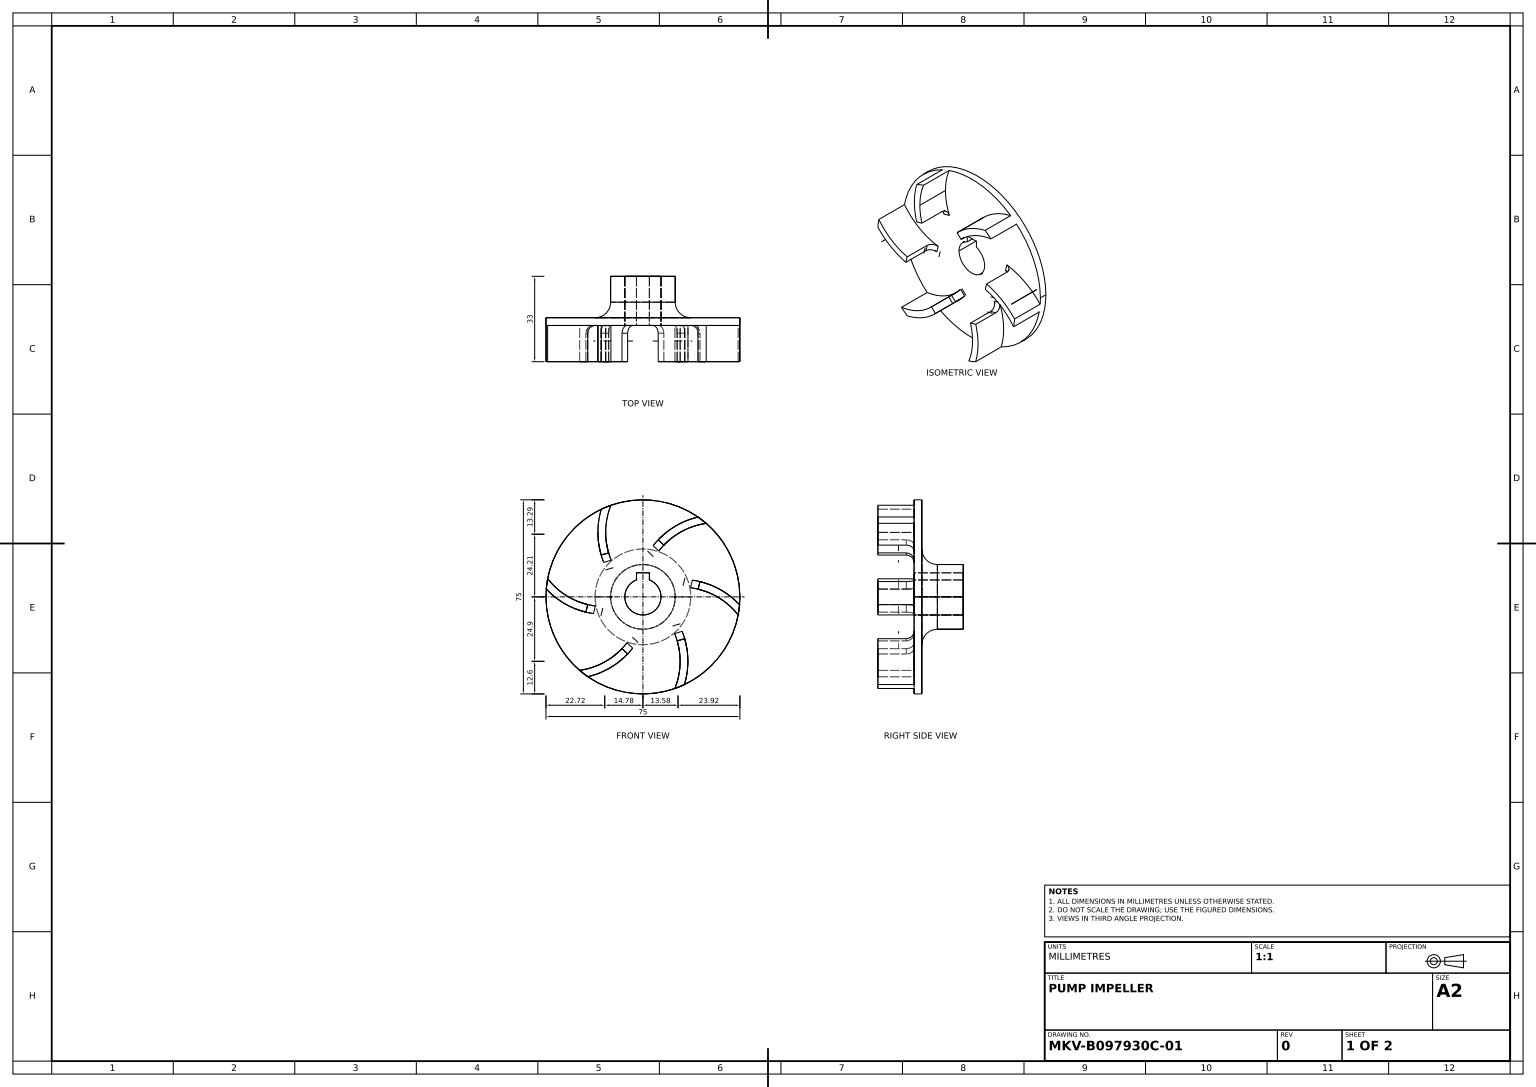
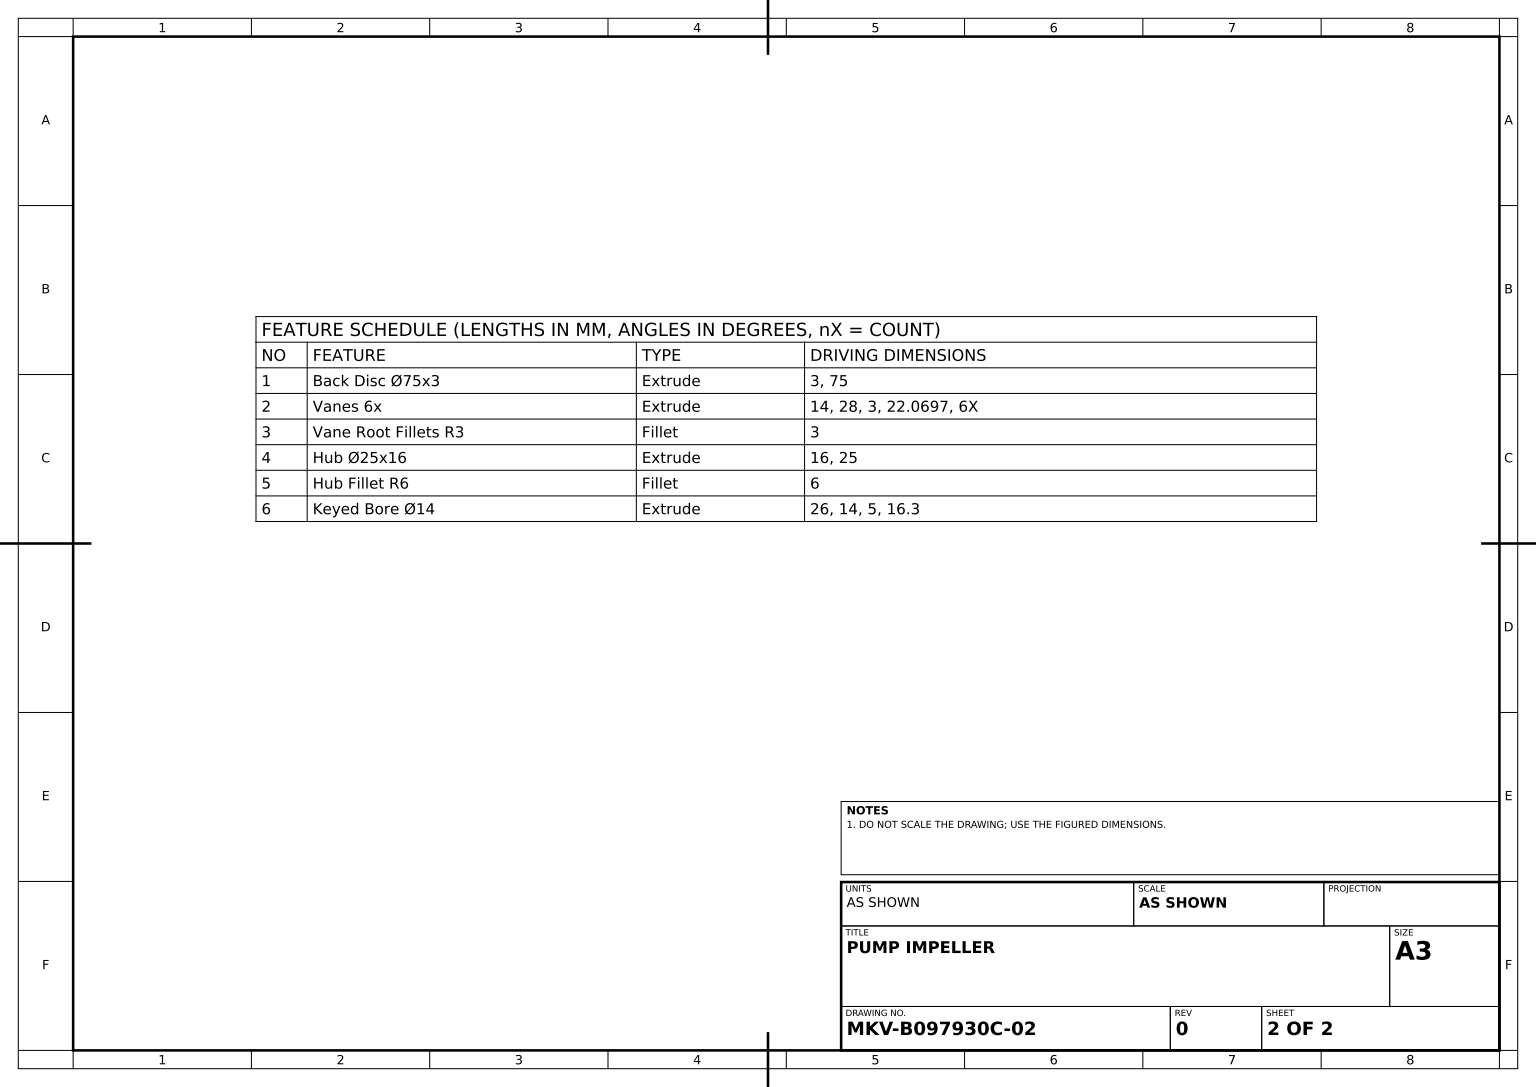
SolidWorks part; units mm, degrees
material "Plain Carbon Steel"
ref_plane "Front Plane" through (0, 0, 0) normal (0, 0, 1) x (1, 0, 0)
ref_plane "Top Plane" through (0, 0, 0) normal (0, 1, 0) x (1, 0, 0)
ref_plane "Right Plane" through (0, 0, 0) normal (1, 0, 0) x (0, 0, -1)
sketch "Back Disc Sketch Ø75" plane through (0, 0, 0) normal (0, 0, 1) x (1, 0, 0)
  line L0 (-142.1179, 0) -> (126.4423, 0) construction
  line L1 (0, 79.4155) -> (0, -87.9448) construction
  circle A0 centre (0, 0) radius 37.5
  dimension "D1" = 75
extrude "Back Disc Ø75x3" add sketch "Back Disc Sketch Ø75" along normal blind 3
sketch "Vane Profiles 6x Sketch" plane through (0, 0, 3) normal (0, 0, 1) x (1, 0, 0)
  line L0 (-50.7637, 0) -> (51.1917, 0) construction
  line L1 (0, 51.3415) -> (0, -56.2417) construction
  line L2 (-21.3637, -3) -> (-22.0697, -5.9158)
  line L3 (-13.2799, 17.0015) -> (-16.158, 16.155)
  line L4 (8.0838, 20.0015) -> (5.9116, 22.0708)
  line L5 (21.3637, 3) -> (22.0697, 5.9158)
  line L6 (13.2799, -17.0015) -> (16.158, -16.155)
  line L7 (-8.0838, -20.0015) -> (-5.9116, -22.0708)
  arc A0 (-37.3798, 3) -> (-22.0697, -5.9158) centre (-14.775, 24.2138) ccw
  circle A1 centre (0, 0) radius 37.5
  arc A2 (-36.8444, 6.9817) -> (-37.3798, 3) centre (0, 0) ccw
  arc A3 (-36.8444, 6.9817) -> (-21.3637, -3) centre (-14.775, 24.2138) ccw
  arc A4 (-12.3759, 35.399) -> (-13.2799, 17.0015) centre (13.5822, 24.9024) ccw
  arc A5 (-39.2089, 5.1354) -> (-22.0697, -5.9158) centre (-14.775, 24.2138) ccw construction
  arc A6 (-16.0918, 33.8719) -> (-16.158, 16.155) centre (13.5822, 24.9024) ccw
  arc A7 (-12.3759, 35.399) -> (-16.0918, 33.8719) centre (0, 0) ccw
  arc A8 (24.4685, 28.4173) -> (8.0838, 20.0015) centre (28.3572, 0.6887) ccw
  arc A9 (21.288, 30.8719) -> (5.9116, 22.0708) centre (28.3572, 0.6887) ccw
  arc A10 (24.4685, 28.4173) -> (21.288, 30.8719) centre (0, 0) ccw
  arc A11 (36.8444, -6.9817) -> (21.3637, 3) centre (14.775, -24.2138) ccw
  arc A12 (37.3798, -3) -> (22.0697, 5.9158) centre (14.775, -24.2138) ccw
  arc A13 (36.8444, -6.9817) -> (37.3798, -3) centre (0, 0) ccw
  arc A14 (12.3759, -35.399) -> (13.2799, -17.0015) centre (-13.5822, -24.9024) ccw
  arc A15 (16.0918, -33.8719) -> (16.158, -16.155) centre (-13.5822, -24.9024) ccw
  arc A16 (12.3759, -35.399) -> (16.0918, -33.8719) centre (0, 0) ccw
  arc A17 (-24.4685, -28.4173) -> (-8.0838, -20.0015) centre (-28.3572, -0.6887) ccw
  arc A18 (-21.288, -30.8719) -> (-5.9116, -22.0708) centre (-28.3572, -0.6887) ccw
  arc A19 (-24.4685, -28.4173) -> (-21.288, -30.8719) centre (0, 0) ccw
  point P46 (0, 0)
  dimension "D2" = 3
  dimension "D4" = 28
  dimension "D3" = 3
  dimension "D5" = 3
  dimension "D6" = 22.0697
  dimension "D1" = 0
  dimension "D7" = 6
extrude "Vanes 6x" add sketch "Vane Profiles 6x Sketch" along normal blind 14
fillet "Vane Root Fillets R3" radius 3 6 edges at (14.719, -16.5783, 3) (-6.9977, -21.0362, 3) (21.7167, 4.4579, 3) (-21.7167, -4.4579, 3) (6.9977, 21.0362, 3) (-14.719, 16.5783, 3)
sketch "Hub Sketch Ø25" plane through (0, 0, 0) normal (0, 0, -1) x (-1, 0, 0)
  circle A0 centre (0, 0) radius 12.5
  dimension "D1" = 25
extrude "Hub Ø25x16" add sketch "Hub Sketch Ø25" along normal blind 16
fillet "Hub Fillet R6" radius 6 1 edges at (-12.5, 0, 0)
sketch "Keyed Bore Sketch Ø14" plane through (0, 0, 3) normal (0, 0, 1) x (1, 0, 0)
  line L0 (0, 15.4541) -> (0, -7) construction
  line L1 (-2.5, 9.3) -> (2.5, 9.3)
  line L2 (-2.5, 9.3) -> (-2.5, 6.5383)
  line L3 (2.5, 9.3) -> (2.5, 6.5383)
  arc A0 (-2.5, 6.5383) -> (2.5, 6.5383) centre (0, 0) ccw
  dimension "D1" = 14
  dimension "D2" = 5
  dimension "D3" = 16.3
extrude "Keyed Bore Ø14" cut sketch "Keyed Bore Sketch Ø14" against normal blind 26
